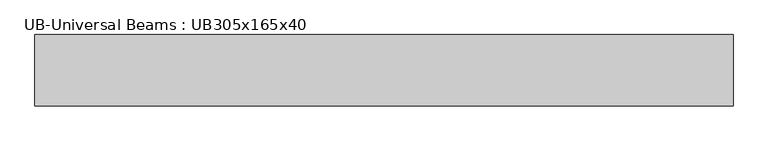
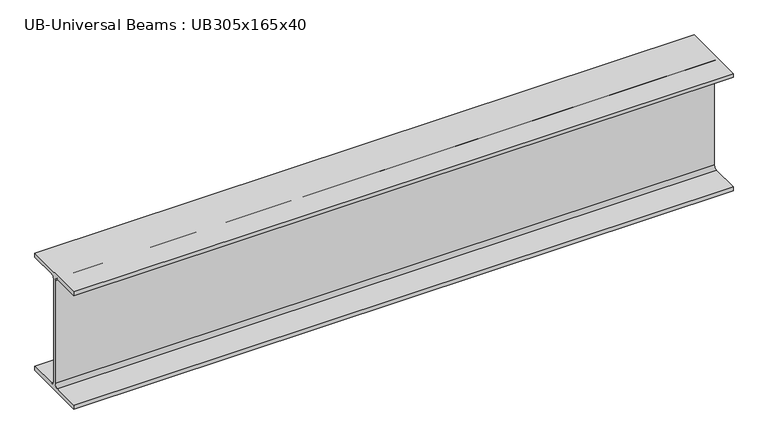
"""IFC4 building model written with IfcOpenShell, lengths in millimetres: beam geometry, UB-Universal Beams : UB305x165x40."""

from ifc_helpers import new_model, si_unit, point, frame, frame_2d, origin, place, context, project, spatial, polyline, circle_curve, trimmed, segment, composite_curve, outline, extrude, source, transform, mapped, element, save


def ub_universal_beams_ub305x165x40_ec3a2bf0(model_context):
    return source(origin(), model_context, "Body", "SweptSolid", [
        extrude(outline(composite_curve([segment(polyline([(82.5, -141.5), (82.5, -151.7), (-82.5, -151.7), (-82.5, -141.5), (-11.9, -141.5)]), True, "CONTINUOUS"), segment(trimmed(circle_curve(frame_2d((-11.9, -132.6)), 8.9), [point((-11.9, -141.5))], [point((-3.0, -132.6))], True, "CARTESIAN"), True, "CONTINUOUS"), segment(polyline([(-3.0, -132.6), (-3.0, 132.6)]), True, "CONTINUOUS"), segment(trimmed(circle_curve(frame_2d((-11.9, 132.6)), 8.9), [point((-3.0, 132.6))], [point((-11.9, 141.5))], True, "CARTESIAN"), True, "CONTINUOUS"), segment(polyline([(-11.9, 141.5), (-82.5, 141.5), (-82.5, 151.7), (82.5, 151.7), (82.5, 141.5), (11.9, 141.5)]), True, "CONTINUOUS"), segment(trimmed(circle_curve(frame_2d((11.9, 132.6)), 8.9), [point((11.9, 141.5))], [point((3.0, 132.6))], True, "CARTESIAN"), True, "CONTINUOUS"), segment(polyline([(3.0, 132.6), (3.0, -132.6)]), True, "CONTINUOUS"), segment(trimmed(circle_curve(frame_2d((11.9, -132.6)), 8.9), [point((3.0, -132.6))], [point((11.9, -141.5))], True, "CARTESIAN"), True, "CONTINUOUS"), segment(polyline([(11.9, -141.5), (82.5, -141.5)]), True, "CONTINUOUS")], self_intersect=False)), frame((-899.35, 0.0, 0.0), z_axis=(1.0, 0.0, 0.0), x_axis=(0.0, 1.0, 0.0)), (0.0, 0.0, 1.0), 1615.0),
    ])


if __name__ == "__main__":
    model = new_model("IFC4")
    model_context = context("Model", 3, world=origin())
    ifc_project = project(units=[si_unit("LENGTHUNIT", "METRE", prefix="MILLI")], contexts=[model_context])
    site = spatial("IfcSite", under=ifc_project)
    building = spatial("IfcBuilding", under=site)
    placement = place(None, origin())
    ub_universal_beams_ub305x165x40_shape = ub_universal_beams_ub305x165x40_ec3a2bf0(model_context)
    element("IfcBeam", 1, ObjectType="UB-Universal Beams : UB305x165x40", at=placement, inside=building, context=model_context, shape_type="MappedRepresentation", body=[
        mapped(ub_universal_beams_ub305x165x40_shape, transform((0.0, 0.0, 0.0), x_axis=(1.0, 0.0, 0.0), y_axis=(0.0, 1.0, 0.0), z_axis=(0.0, 0.0, 1.0))),
    ])
    save(model, "model.ifc")

# Revit data of these elements
# Type "UB-Universal Beams : UB305x165x40"
#   Section Name Key = "UB305X165X40"
#   Width = 16.5 cm
#   Web Thickness = 0.6 cm
#   Web Fillet = 0.89 cm
#   Warping Constant = 164000.0 cm⁶
#   Torsional Moment of Inertia = 14.70 cm⁴
#   Section Area = 51.3 cm²
#   Plastic Modulus weak axis = 142.0 cm³
#   Plastic Modulus strong axis = 623.0 cm³
#   Nominal Weight = 40.2999 kgf/m
#   Moment of Inertia weak axis = 764.00 cm⁴
#   Moment of Inertia strong axis = 8503.00 cm⁴
#   Height = 30.34 cm
#   Flange Thickness = 1.02 cm
#   Elastic Modulus weak axis = 92.6 cm³
#   Elastic Modulus strong axis = 560.0 cm³
#   Centroid Vertical = 15.17 cm
#   Centroid Horizontal = 8.25 cm
#   Bolt Spacing = 9.0 cm
#   Length [instance default] = 1500 mm
#   Structural Material [instance default] = Metal - Steel 43-275
#   Type Comments = ""
#   Assembly Code = ""
# Element 1 (IfcBeam, "UB-Universal Beams : UB305x165x40")
#   Materials on its faces: "Metal - Steel 43-275"
# Materials
#   "Metal - Steel 43-275": class "Metal", colour RGB 247 247 247, transparency 0, Cost = 0
